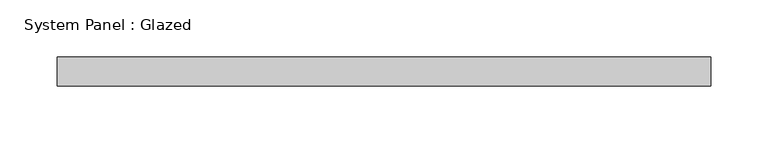
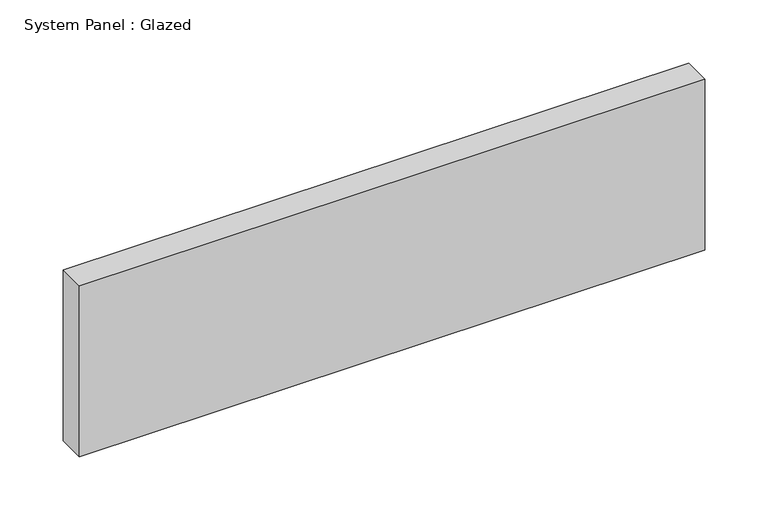
"""IFC4 building model written with IfcOpenShell, lengths in millimetres: plate geometry, System Panel : Glazed."""

from ifc_helpers import new_model, si_unit, origin, origin_with_axes, place, context, project, spatial, polyline, outline, extrude, source, transform, mapped, element, save


def system_panel_glazed_23b8b45c(model_context):
    return source(origin(), model_context, "Body", "SweptSolid", [
        extrude(outline(polyline([(285.75, 19.05), (-285.75, 19.05), (-285.75, 44.45), (285.75, 44.45), (285.75, 19.05)])), origin_with_axes(), (0.0, 0.0, 1.0), 165.1),
    ])


if __name__ == "__main__":
    model = new_model("IFC4")
    model_context = context("Model", 3, world=origin())
    ifc_project = project(units=[si_unit("LENGTHUNIT", "METRE", prefix="MILLI")], contexts=[model_context])
    site = spatial("IfcSite", under=ifc_project)
    building = spatial("IfcBuilding", under=site)
    placement = place(None, origin())
    system_panel_glazed_shape = system_panel_glazed_23b8b45c(model_context)
    element("IfcPlate", 1, ObjectType="System Panel : Glazed", at=placement, inside=building, context=model_context, shape_type="MappedRepresentation", body=[
        mapped(system_panel_glazed_shape, transform((0.0, 0.0, 0.0), x_axis=(1.0, 0.0, 0.0), y_axis=(0.0, 1.0, 0.0), z_axis=(0.0, 0.0, 1.0))),
    ])
    save(model, "model.ifc")

# Revit data of these elements
# Type "System Panel : Glazed"
#   Construction Type Id = "GSP4R"
#   Analytic Construction = "1/8 in Pilkington single glazing"
#   Visual Light Transmittance = 0.9
#   Solar Heat Gain Coefficient = 0.86
#   Heat Transfer Coefficient (U) = 1.18115 BTU/(h·ft²·°F)
#   Define Thermal Properties by = 1
# Element 1 (IfcPlate, "System Panel : Glazed")
#   Materials on its faces: "Glass"
# Materials
#   "Glass": class "Glass", colour RGB 0 128 192, transparency 0.75, Description = "Soda Lime Glass", Cost = 0
